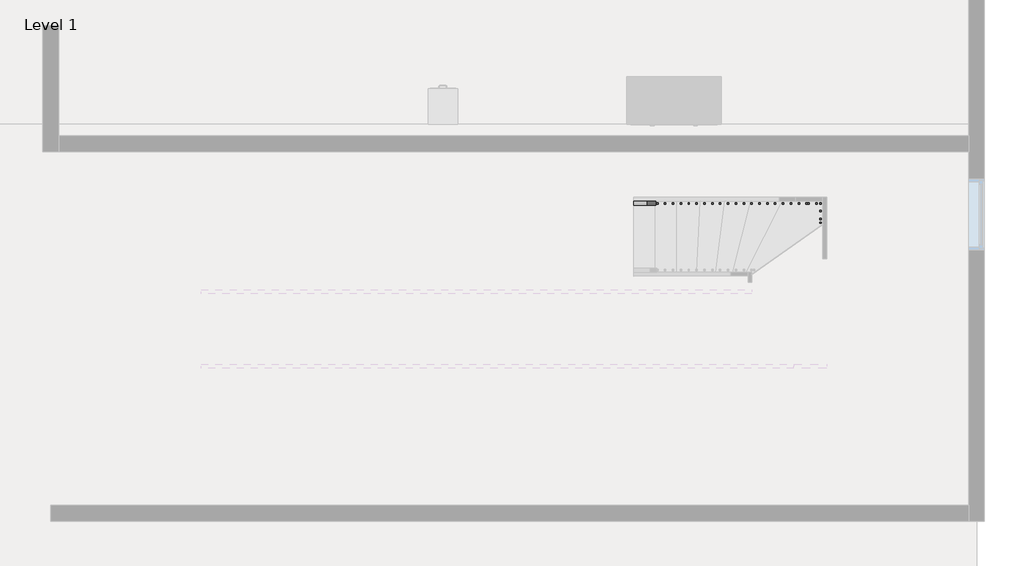
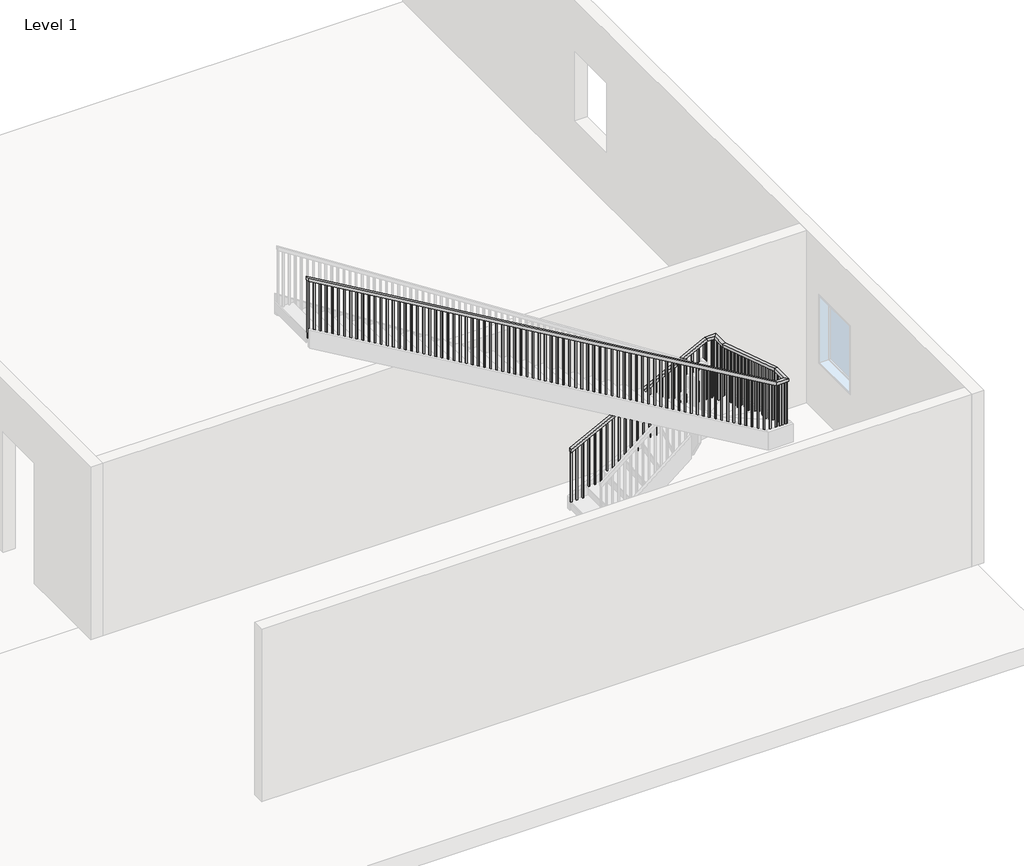
# One storey, part 3 of 4: 1 railing.
"""IFC4 building model written with IfcOpenShell, lengths in millimetres."""

from ifc_helpers import new_model, si_unit, frame, origin, place, context, project, spatial, polyline, outline, extrude, faceted_brep, element, save

model = new_model("IFC4")

# Units and contexts
model_context = context("Model", 3, world=origin())
ifc_project = project(units=[si_unit("LENGTHUNIT", "METRE", prefix="MILLI")], contexts=[model_context])

# Site, building, storey
site = spatial("IfcSite", under=ifc_project)
building = spatial("IfcBuilding", under=site)
storey = spatial("IfcBuildingStorey", under=building, Name="Level 1", Elevation=0.0)

# Railing
placement = place(None, origin())
element("IfcRailing", 1, ObjectType="Handrail - Rectangular", at=placement, inside=storey, context=model_context, shape_type="SolidModel", body=[
    faceted_brep([(11576.2992414, 971.4275916, 1109.0771751), (11576.2992414, 971.4275916, 1051.9280057), (11576.2992414, 920.6275916, 1051.9280057), (11576.2992414, 920.6275916, 1109.0771751), (13836.2810979, 971.4275916, 2273.7644996), (13848.6011492, 971.4275916, 2222.9644996), (13848.6011492, 920.6275916, 2222.9644996), (13836.2810979, 920.6275916, 2273.7644996), (14018.4309332, 971.4275916, 2273.7644996), (14018.4309332, 971.4275916, 2222.9644996), (13967.6309332, 920.6275916, 2222.9644996), (13967.6309332, 920.6275916, 2273.7644996), (14018.4309332, 694.273639, 2273.7644996), (14018.4309332, 686.3230629, 2222.9644996), (13967.6309332, 686.3230629, 2222.9644996), (13967.6309332, 694.273639, 2273.7644996), (14018.4309332, -805.6099604, 2755.0388853), (14018.4309332, -813.5605365, 2704.2388853), (13967.6309332, -813.5605365, 2704.2388853), (13967.6309332, -805.6099604, 2755.0388853), (14018.4309332, -1136.7724084, 2704.2388853), (14018.4309332, -1136.7724084, 2755.0388853), (13825.4484846, -1136.7724084, 2755.0388853), (13811.671706, -1136.7724084, 2704.2388853), (13967.6309332, -1085.9724084, 2704.2388853), (13811.671706, -1085.9724084, 2704.2388853), (13967.6309332, -1085.9724084, 2755.0388853), (13825.4484846, -1085.9724084, 2755.0388853), (5988.2992414, -1136.7724084, 7343.3084387), (5988.2992414, -1085.9724084, 7343.3084387), (5988.2992414, -1085.9724084, 7284.4428051), (5988.2992414, -1136.7724084, 7284.4428051)], [[[0, 1, 2, 3]], [[1, 0, 4, 5]], [[2, 1, 5, 6]], [[3, 2, 6, 7]], [[0, 3, 7, 4]], [[5, 4, 8, 9]], [[6, 5, 9, 10]], [[7, 6, 10, 11]], [[4, 7, 11, 8]], [[9, 8, 12, 13]], [[10, 9, 13, 14]], [[11, 10, 14, 15]], [[8, 11, 15, 12]], [[13, 12, 16, 17]], [[14, 13, 17, 18]], [[15, 14, 18, 19]], [[12, 15, 19, 16]], [[20, 21, 22, 23]], [[24, 20, 23, 25]], [[26, 24, 25, 27]], [[21, 26, 27, 22]], [[17, 16, 21, 20]], [[18, 17, 20, 24]], [[19, 18, 24, 26]], [[16, 19, 26, 21]], [[28, 29, 30, 31]], [[23, 22, 28, 31]], [[25, 23, 31, 30]], [[27, 25, 30, 29]], [[22, 27, 29, 28]]]),
    extrude(outline(polyline([(7281.852626, 5992.7234846), (6265.3333333, 5992.7234846), (6265.3333333, 6011.7734846), (7270.6997779, 6011.7734846), (7281.852626, 5992.7234846)])), frame((0.0, -1120.8974084, 0.0), z_axis=(0.0, 1.0, 0.0), x_axis=(0.0, 0.0, 1.0)), (0.0, 0.0, 1.0), 19.05),
    extrude(outline(polyline([(7222.3707695, 6094.3234846), (6265.3333333, 6094.3234846), (6265.3333333, 6113.3734846), (7211.2179214, 6113.3734846), (7222.3707695, 6094.3234846)])), frame((0.0, -1120.8974084, 0.0), z_axis=(0.0, 1.0, 0.0), x_axis=(0.0, 0.0, 1.0)), (0.0, 0.0, 1.0), 19.05),
    extrude(outline(polyline([(7162.888913, 6195.9234846), (6265.3333333, 6195.9234846), (6265.3333333, 6214.9734846), (7151.7360649, 6214.9734846), (7162.888913, 6195.9234846)])), frame((0.0, -1120.8974084, 0.0), z_axis=(0.0, 1.0, 0.0), x_axis=(0.0, 0.0, 1.0)), (0.0, 0.0, 1.0), 19.05),
    extrude(outline(polyline([(7103.4070565, 6297.5234846), (6096.0, 6297.5234846), (6096.0, 6316.5734846), (7092.2542084, 6316.5734846), (7103.4070565, 6297.5234846)])), frame((0.0, -1120.8974084, 0.0), z_axis=(0.0, 1.0, 0.0), x_axis=(0.0, 0.0, 1.0)), (0.0, 0.0, 1.0), 19.05),
    extrude(outline(polyline([(7043.9252, 6399.1234846), (6096.0, 6399.1234846), (6096.0, 6418.1734846), (7032.7723519, 6418.1734846), (7043.9252, 6399.1234846)])), frame((0.0, -1120.8974084, 0.0), z_axis=(0.0, 1.0, 0.0), x_axis=(0.0, 0.0, 1.0)), (0.0, 0.0, 1.0), 19.05),
    extrude(outline(polyline([(6984.4433435, 6500.7234846), (6096.0, 6500.7234846), (6096.0, 6519.7734846), (6973.2904954, 6519.7734846), (6984.4433435, 6500.7234846)])), frame((0.0, -1120.8974084, 0.0), z_axis=(0.0, 1.0, 0.0), x_axis=(0.0, 0.0, 1.0)), (0.0, 0.0, 1.0), 19.05),
    extrude(outline(polyline([(6924.961487, 6602.3234846), (5926.6666667, 6602.3234846), (5926.6666667, 6621.3734846), (6913.8086389, 6621.3734846), (6924.961487, 6602.3234846)])), frame((0.0, -1120.8974084, 0.0), z_axis=(0.0, 1.0, 0.0), x_axis=(0.0, 0.0, 1.0)), (0.0, 0.0, 1.0), 19.05),
    extrude(outline(polyline([(6865.4796305, 6703.9234846), (5926.6666667, 6703.9234846), (5926.6666667, 6722.9734846), (6854.3267824, 6722.9734846), (6865.4796305, 6703.9234846)])), frame((0.0, -1120.8974084, 0.0), z_axis=(0.0, 1.0, 0.0), x_axis=(0.0, 0.0, 1.0)), (0.0, 0.0, 1.0), 19.05),
    extrude(outline(polyline([(6805.997774, 6805.5234846), (5926.6666667, 6805.5234846), (5926.6666667, 6824.5734846), (6794.8449259, 6824.5734846), (6805.997774, 6805.5234846)])), frame((0.0, -1120.8974084, 0.0), z_axis=(0.0, 1.0, 0.0), x_axis=(0.0, 0.0, 1.0)), (0.0, 0.0, 1.0), 19.05),
    extrude(outline(polyline([(6746.5159175, 6907.1234846), (5757.3333333, 6907.1234846), (5757.3333333, 6926.1734846), (6735.3630694, 6926.1734846), (6746.5159175, 6907.1234846)])), frame((0.0, -1120.8974084, 0.0), z_axis=(0.0, 1.0, 0.0), x_axis=(0.0, 0.0, 1.0)), (0.0, 0.0, 1.0), 19.05),
    extrude(outline(polyline([(6687.034061, 7008.7234846), (5757.3333333, 7008.7234846), (5757.3333333, 7027.7734846), (6675.881213, 7027.7734846), (6687.034061, 7008.7234846)])), frame((0.0, -1120.8974084, 0.0), z_axis=(0.0, 1.0, 0.0), x_axis=(0.0, 0.0, 1.0)), (0.0, 0.0, 1.0), 19.05),
    extrude(outline(polyline([(6627.5522045, 7110.3234846), (5588.0, 7110.3234846), (5588.0, 7129.3734846), (6616.3993565, 7129.3734846), (6627.5522045, 7110.3234846)])), frame((0.0, -1120.8974084, 0.0), z_axis=(0.0, 1.0, 0.0), x_axis=(0.0, 0.0, 1.0)), (0.0, 0.0, 1.0), 19.05),
    extrude(outline(polyline([(6568.0703481, 7211.9234846), (5588.0, 7211.9234846), (5588.0, 7230.9734846), (6556.9175, 7230.9734846), (6568.0703481, 7211.9234846)])), frame((0.0, -1120.8974084, 0.0), z_axis=(0.0, 1.0, 0.0), x_axis=(0.0, 0.0, 1.0)), (0.0, 0.0, 1.0), 19.05),
    extrude(outline(polyline([(6508.5884916, 7313.5234846), (5588.0, 7313.5234846), (5588.0, 7332.5734846), (6497.4356435, 7332.5734846), (6508.5884916, 7313.5234846)])), frame((0.0, -1120.8974084, 0.0), z_axis=(0.0, 1.0, 0.0), x_axis=(0.0, 0.0, 1.0)), (0.0, 0.0, 1.0), 19.05),
    extrude(outline(polyline([(6449.1066351, 7415.1234846), (5418.6666667, 7415.1234846), (5418.6666667, 7434.1734846), (6437.953787, 7434.1734846), (6449.1066351, 7415.1234846)])), frame((0.0, -1120.8974084, 0.0), z_axis=(0.0, 1.0, 0.0), x_axis=(0.0, 0.0, 1.0)), (0.0, 0.0, 1.0), 19.05),
    extrude(outline(polyline([(6389.6247786, 7516.7234846), (5418.6666667, 7516.7234846), (5418.6666667, 7535.7734846), (6378.4719305, 7535.7734846), (6389.6247786, 7516.7234846)])), frame((0.0, -1120.8974084, 0.0), z_axis=(0.0, 1.0, 0.0), x_axis=(0.0, 0.0, 1.0)), (0.0, 0.0, 1.0), 19.05),
    extrude(outline(polyline([(6330.1429221, 7618.3234846), (5418.6666667, 7618.3234846), (5418.6666667, 7637.3734846), (6318.990074, 7637.3734846), (6330.1429221, 7618.3234846)])), frame((0.0, -1120.8974084, 0.0), z_axis=(0.0, 1.0, 0.0), x_axis=(0.0, 0.0, 1.0)), (0.0, 0.0, 1.0), 19.05),
    extrude(outline(polyline([(6270.6610656, 7719.9234846), (5249.3333333, 7719.9234846), (5249.3333333, 7738.9734846), (6259.5082175, 7738.9734846), (6270.6610656, 7719.9234846)])), frame((0.0, -1120.8974084, 0.0), z_axis=(0.0, 1.0, 0.0), x_axis=(0.0, 0.0, 1.0)), (0.0, 0.0, 1.0), 19.05),
    extrude(outline(polyline([(6211.1792091, 7821.5234846), (5249.3333333, 7821.5234846), (5249.3333333, 7840.5734846), (6200.026361, 7840.5734846), (6211.1792091, 7821.5234846)])), frame((0.0, -1120.8974084, 0.0), z_axis=(0.0, 1.0, 0.0), x_axis=(0.0, 0.0, 1.0)), (0.0, 0.0, 1.0), 19.05),
    extrude(outline(polyline([(6151.6973526, 7923.1234846), (5249.3333333, 7923.1234846), (5249.3333333, 7942.1734846), (6140.5445045, 7942.1734846), (6151.6973526, 7923.1234846)])), frame((0.0, -1120.8974084, 0.0), z_axis=(0.0, 1.0, 0.0), x_axis=(0.0, 0.0, 1.0)), (0.0, 0.0, 1.0), 19.05),
    extrude(outline(polyline([(6092.2154961, 8024.7234846), (5080.0, 8024.7234846), (5080.0, 8043.7734846), (6081.062648, 8043.7734846), (6092.2154961, 8024.7234846)])), frame((0.0, -1120.8974084, 0.0), z_axis=(0.0, 1.0, 0.0), x_axis=(0.0, 0.0, 1.0)), (0.0, 0.0, 1.0), 19.05),
    extrude(outline(polyline([(6032.7336396, 8126.3234846), (5080.0, 8126.3234846), (5080.0, 8145.3734846), (6021.5807915, 8145.3734846), (6032.7336396, 8126.3234846)])), frame((0.0, -1120.8974084, 0.0), z_axis=(0.0, 1.0, 0.0), x_axis=(0.0, 0.0, 1.0)), (0.0, 0.0, 1.0), 19.05),
    extrude(outline(polyline([(5973.2517831, 8227.9234846), (4910.6666667, 8227.9234846), (4910.6666667, 8246.9734846), (5962.098935, 8246.9734846), (5973.2517831, 8227.9234846)])), frame((0.0, -1120.8974084, 0.0), z_axis=(0.0, 1.0, 0.0), x_axis=(0.0, 0.0, 1.0)), (0.0, 0.0, 1.0), 19.05),
    extrude(outline(polyline([(5913.7699266, 8329.5234846), (4910.6666667, 8329.5234846), (4910.6666667, 8348.5734846), (5902.6170785, 8348.5734846), (5913.7699266, 8329.5234846)])), frame((0.0, -1120.8974084, 0.0), z_axis=(0.0, 1.0, 0.0), x_axis=(0.0, 0.0, 1.0)), (0.0, 0.0, 1.0), 19.05),
    extrude(outline(polyline([(5854.2880701, 8431.1234846), (4910.6666667, 8431.1234846), (4910.6666667, 8450.1734846), (5843.135222, 8450.1734846), (5854.2880701, 8431.1234846)])), frame((0.0, -1120.8974084, 0.0), z_axis=(0.0, 1.0, 0.0), x_axis=(0.0, 0.0, 1.0)), (0.0, 0.0, 1.0), 19.05),
    extrude(outline(polyline([(5794.8062136, 8532.7234846), (4741.3333333, 8532.7234846), (4741.3333333, 8551.7734846), (5783.6533655, 8551.7734846), (5794.8062136, 8532.7234846)])), frame((0.0, -1120.8974084, 0.0), z_axis=(0.0, 1.0, 0.0), x_axis=(0.0, 0.0, 1.0)), (0.0, 0.0, 1.0), 19.05),
    extrude(outline(polyline([(5735.3243571, 8634.3234846), (4741.3333333, 8634.3234846), (4741.3333333, 8653.3734846), (5724.171509, 8653.3734846), (5735.3243571, 8634.3234846)])), frame((0.0, -1120.8974084, 0.0), z_axis=(0.0, 1.0, 0.0), x_axis=(0.0, 0.0, 1.0)), (0.0, 0.0, 1.0), 19.05),
    extrude(outline(polyline([(5675.8425006, 8735.9234846), (4741.3333333, 8735.9234846), (4741.3333333, 8754.9734846), (5664.6896525, 8754.9734846), (5675.8425006, 8735.9234846)])), frame((0.0, -1120.8974084, 0.0), z_axis=(0.0, 1.0, 0.0), x_axis=(0.0, 0.0, 1.0)), (0.0, 0.0, 1.0), 19.05),
    extrude(outline(polyline([(5616.3606441, 8837.5234846), (4572.0, 8837.5234846), (4572.0, 8856.5734846), (5605.207796, 8856.5734846), (5616.3606441, 8837.5234846)])), frame((0.0, -1120.8974084, 0.0), z_axis=(0.0, 1.0, 0.0), x_axis=(0.0, 0.0, 1.0)), (0.0, 0.0, 1.0), 19.05),
    extrude(outline(polyline([(5556.8787876, 8939.1234846), (4572.0, 8939.1234846), (4572.0, 8958.1734846), (5545.7259395, 8958.1734846), (5556.8787876, 8939.1234846)])), frame((0.0, -1120.8974084, 0.0), z_axis=(0.0, 1.0, 0.0), x_axis=(0.0, 0.0, 1.0)), (0.0, 0.0, 1.0), 19.05),
    extrude(outline(polyline([(5497.3969311, 9040.7234846), (4572.0, 9040.7234846), (4572.0, 9059.7734846), (5486.244083, 9059.7734846), (5497.3969311, 9040.7234846)])), frame((0.0, -1120.8974084, 0.0), z_axis=(0.0, 1.0, 0.0), x_axis=(0.0, 0.0, 1.0)), (0.0, 0.0, 1.0), 19.05),
    extrude(outline(polyline([(5437.9150746, 9142.3234846), (4402.6666667, 9142.3234846), (4402.6666667, 9161.3734846), (5426.7622265, 9161.3734846), (5437.9150746, 9142.3234846)])), frame((0.0, -1120.8974084, 0.0), z_axis=(0.0, 1.0, 0.0), x_axis=(0.0, 0.0, 1.0)), (0.0, 0.0, 1.0), 19.05),
    extrude(outline(polyline([(5378.4332181, 9243.9234846), (4402.6666667, 9243.9234846), (4402.6666667, 9262.9734846), (5367.28037, 9262.9734846), (5378.4332181, 9243.9234846)])), frame((0.0, -1120.8974084, 0.0), z_axis=(0.0, 1.0, 0.0), x_axis=(0.0, 0.0, 1.0)), (0.0, 0.0, 1.0), 19.05),
    extrude(outline(polyline([(5318.9513616, 9345.5234846), (4233.3333333, 9345.5234846), (4233.3333333, 9364.5734846), (5307.7985135, 9364.5734846), (5318.9513616, 9345.5234846)])), frame((0.0, -1120.8974084, 0.0), z_axis=(0.0, 1.0, 0.0), x_axis=(0.0, 0.0, 1.0)), (0.0, 0.0, 1.0), 19.05),
    extrude(outline(polyline([(5259.4695051, 9447.1234846), (4233.3333333, 9447.1234846), (4233.3333333, 9466.1734846), (5248.316657, 9466.1734846), (5259.4695051, 9447.1234846)])), frame((0.0, -1120.8974084, 0.0), z_axis=(0.0, 1.0, 0.0), x_axis=(0.0, 0.0, 1.0)), (0.0, 0.0, 1.0), 19.05),
    extrude(outline(polyline([(5199.9876486, 9548.7234846), (4233.3333333, 9548.7234846), (4233.3333333, 9567.7734846), (5188.8348005, 9567.7734846), (5199.9876486, 9548.7234846)])), frame((0.0, -1120.8974084, 0.0), z_axis=(0.0, 1.0, 0.0), x_axis=(0.0, 0.0, 1.0)), (0.0, 0.0, 1.0), 19.05),
    extrude(outline(polyline([(5140.5057921, 9650.3234846), (4064.0, 9650.3234846), (4064.0, 9669.3734846), (5129.352944, 9669.3734846), (5140.5057921, 9650.3234846)])), frame((0.0, -1120.8974084, 0.0), z_axis=(0.0, 1.0, 0.0), x_axis=(0.0, 0.0, 1.0)), (0.0, 0.0, 1.0), 19.05),
    extrude(outline(polyline([(5081.0239356, 9751.9234846), (4064.0, 9751.9234846), (4064.0, 9770.9734846), (5069.8710875, 9770.9734846), (5081.0239356, 9751.9234846)])), frame((0.0, -1120.8974084, 0.0), z_axis=(0.0, 1.0, 0.0), x_axis=(0.0, 0.0, 1.0)), (0.0, 0.0, 1.0), 19.05),
    extrude(outline(polyline([(5021.5420791, 9853.5234846), (4064.0, 9853.5234846), (4064.0, 9872.5734846), (5010.389231, 9872.5734846), (5021.5420791, 9853.5234846)])), frame((0.0, -1120.8974084, 0.0), z_axis=(0.0, 1.0, 0.0), x_axis=(0.0, 0.0, 1.0)), (0.0, 0.0, 1.0), 19.05),
    extrude(outline(polyline([(4962.0602226, 9955.1234846), (3894.6666667, 9955.1234846), (3894.6666667, 9974.1734846), (4950.9073745, 9974.1734846), (4962.0602226, 9955.1234846)])), frame((0.0, -1120.8974084, 0.0), z_axis=(0.0, 1.0, 0.0), x_axis=(0.0, 0.0, 1.0)), (0.0, 0.0, 1.0), 19.05),
    extrude(outline(polyline([(4902.5783661, 10056.7234846), (3894.6666667, 10056.7234846), (3894.6666667, 10075.7734846), (4891.4255181, 10075.7734846), (4902.5783661, 10056.7234846)])), frame((0.0, -1120.8974084, 0.0), z_axis=(0.0, 1.0, 0.0), x_axis=(0.0, 0.0, 1.0)), (0.0, 0.0, 1.0), 19.05),
    extrude(outline(polyline([(4843.0965096, 10158.3234846), (3894.6666667, 10158.3234846), (3894.6666667, 10177.3734846), (4831.9436616, 10177.3734846), (4843.0965096, 10158.3234846)])), frame((0.0, -1120.8974084, 0.0), z_axis=(0.0, 1.0, 0.0), x_axis=(0.0, 0.0, 1.0)), (0.0, 0.0, 1.0), 19.05),
    extrude(outline(polyline([(4783.6146532, 10259.9234846), (3725.3333333, 10259.9234846), (3725.3333333, 10278.9734846), (4772.4618051, 10278.9734846), (4783.6146532, 10259.9234846)])), frame((0.0, -1120.8974084, 0.0), z_axis=(0.0, 1.0, 0.0), x_axis=(0.0, 0.0, 1.0)), (0.0, 0.0, 1.0), 19.05),
    extrude(outline(polyline([(4724.1327967, 10361.5234846), (3725.3333333, 10361.5234846), (3725.3333333, 10380.5734846), (4712.9799486, 10380.5734846), (4724.1327967, 10361.5234846)])), frame((0.0, -1120.8974084, 0.0), z_axis=(0.0, 1.0, 0.0), x_axis=(0.0, 0.0, 1.0)), (0.0, 0.0, 1.0), 19.05),
    extrude(outline(polyline([(4664.6509402, 10463.1234846), (3725.3333333, 10463.1234846), (3725.3333333, 10482.1734846), (4653.4980921, 10482.1734846), (4664.6509402, 10463.1234846)])), frame((0.0, -1120.8974084, 0.0), z_axis=(0.0, 1.0, 0.0), x_axis=(0.0, 0.0, 1.0)), (0.0, 0.0, 1.0), 19.05),
    extrude(outline(polyline([(4605.1690837, 10564.7234846), (3556.0, 10564.7234846), (3556.0, 10583.7734846), (4594.0162356, 10583.7734846), (4605.1690837, 10564.7234846)])), frame((0.0, -1120.8974084, 0.0), z_axis=(0.0, 1.0, 0.0), x_axis=(0.0, 0.0, 1.0)), (0.0, 0.0, 1.0), 19.05),
    extrude(outline(polyline([(4545.6872272, 10666.3234846), (3556.0, 10666.3234846), (3556.0, 10685.3734846), (4534.5343791, 10685.3734846), (4545.6872272, 10666.3234846)])), frame((0.0, -1120.8974084, 0.0), z_axis=(0.0, 1.0, 0.0), x_axis=(0.0, 0.0, 1.0)), (0.0, 0.0, 1.0), 19.05),
    extrude(outline(polyline([(4486.2053707, 10767.9234846), (3386.6666667, 10767.9234846), (3386.6666667, 10786.9734846), (4475.0525226, 10786.9734846), (4486.2053707, 10767.9234846)])), frame((0.0, -1120.8974084, 0.0), z_axis=(0.0, 1.0, 0.0), x_axis=(0.0, 0.0, 1.0)), (0.0, 0.0, 1.0), 19.05),
    extrude(outline(polyline([(4426.7235142, 10869.5234846), (3386.6666667, 10869.5234846), (3386.6666667, 10888.5734846), (4415.5706661, 10888.5734846), (4426.7235142, 10869.5234846)])), frame((0.0, -1120.8974084, 0.0), z_axis=(0.0, 1.0, 0.0), x_axis=(0.0, 0.0, 1.0)), (0.0, 0.0, 1.0), 19.05),
    extrude(outline(polyline([(4367.2416577, 10971.1234846), (3386.6666667, 10971.1234846), (3386.6666667, 10990.1734846), (4356.0888096, 10990.1734846), (4367.2416577, 10971.1234846)])), frame((0.0, -1120.8974084, 0.0), z_axis=(0.0, 1.0, 0.0), x_axis=(0.0, 0.0, 1.0)), (0.0, 0.0, 1.0), 19.05),
    extrude(outline(polyline([(4307.7598012, 11072.7234846), (3217.3333333, 11072.7234846), (3217.3333333, 11091.7734846), (4296.6069531, 11091.7734846), (4307.7598012, 11072.7234846)])), frame((0.0, -1120.8974084, 0.0), z_axis=(0.0, 1.0, 0.0), x_axis=(0.0, 0.0, 1.0)), (0.0, 0.0, 1.0), 19.05),
    extrude(outline(polyline([(4248.2779447, 11174.3234846), (3217.3333333, 11174.3234846), (3217.3333333, 11193.3734846), (4237.1250966, 11193.3734846), (4248.2779447, 11174.3234846)])), frame((0.0, -1120.8974084, 0.0), z_axis=(0.0, 1.0, 0.0), x_axis=(0.0, 0.0, 1.0)), (0.0, 0.0, 1.0), 19.05),
    extrude(outline(polyline([(4188.7960882, 11275.9234846), (3217.3333333, 11275.9234846), (3217.3333333, 11294.9734846), (4177.6432401, 11294.9734846), (4188.7960882, 11275.9234846)])), frame((0.0, -1120.8974084, 0.0), z_axis=(0.0, 1.0, 0.0), x_axis=(0.0, 0.0, 1.0)), (0.0, 0.0, 1.0), 19.05),
    extrude(outline(polyline([(4129.3142317, 11377.5234846), (3048.0, 11377.5234846), (3048.0, 11396.5734846), (4118.1613836, 11396.5734846), (4129.3142317, 11377.5234846)])), frame((0.0, -1120.8974084, 0.0), z_axis=(0.0, 1.0, 0.0), x_axis=(0.0, 0.0, 1.0)), (0.0, 0.0, 1.0), 19.05),
    extrude(outline(polyline([(4069.8323752, 11479.1234846), (3048.0, 11479.1234846), (3048.0, 11498.1734846), (4058.6795271, 11498.1734846), (4069.8323752, 11479.1234846)])), frame((0.0, -1120.8974084, 0.0), z_axis=(0.0, 1.0, 0.0), x_axis=(0.0, 0.0, 1.0)), (0.0, 0.0, 1.0), 19.05),
    extrude(outline(polyline([(4010.3505187, 11580.7234846), (3048.0, 11580.7234846), (3048.0, 11599.7734846), (3999.1976706, 11599.7734846), (4010.3505187, 11580.7234846)])), frame((0.0, -1120.8974084, 0.0), z_axis=(0.0, 1.0, 0.0), x_axis=(0.0, 0.0, 1.0)), (0.0, 0.0, 1.0), 19.05),
    extrude(outline(polyline([(3950.8686622, 11682.3234846), (2878.6666667, 11682.3234846), (2878.6666667, 11701.3734846), (3939.7158141, 11701.3734846), (3950.8686622, 11682.3234846)])), frame((0.0, -1120.8974084, 0.0), z_axis=(0.0, 1.0, 0.0), x_axis=(0.0, 0.0, 1.0)), (0.0, 0.0, 1.0), 19.05),
    extrude(outline(polyline([(3891.3868057, 11783.9234846), (2878.6666667, 11783.9234846), (2878.6666667, 11802.9734846), (3880.2339576, 11802.9734846), (3891.3868057, 11783.9234846)])), frame((0.0, -1120.8974084, 0.0), z_axis=(0.0, 1.0, 0.0), x_axis=(0.0, 0.0, 1.0)), (0.0, 0.0, 1.0), 19.05),
    extrude(outline(polyline([(3831.9049492, 11885.5234846), (2878.6666667, 11885.5234846), (2878.6666667, 11904.5734846), (3820.7521011, 11904.5734846), (3831.9049492, 11885.5234846)])), frame((0.0, -1120.8974084, 0.0), z_axis=(0.0, 1.0, 0.0), x_axis=(0.0, 0.0, 1.0)), (0.0, 0.0, 1.0), 19.05),
    extrude(outline(polyline([(3772.4230927, 11987.1234846), (2709.3333333, 11987.1234846), (2709.3333333, 12006.1734846), (3761.2702446, 12006.1734846), (3772.4230927, 11987.1234846)])), frame((0.0, -1120.8974084, 0.0), z_axis=(0.0, 1.0, 0.0), x_axis=(0.0, 0.0, 1.0)), (0.0, 0.0, 1.0), 19.05),
    extrude(outline(polyline([(3712.9412362, 12088.7234846), (2709.3333333, 12088.7234846), (2709.3333333, 12107.7734846), (3701.7883881, 12107.7734846), (3712.9412362, 12088.7234846)])), frame((0.0, -1120.8974084, 0.0), z_axis=(0.0, 1.0, 0.0), x_axis=(0.0, 0.0, 1.0)), (0.0, 0.0, 1.0), 19.05),
    extrude(outline(polyline([(3653.4593797, 12190.3234846), (2540.0, 12190.3234846), (2540.0, 12209.3734846), (3642.3065316, 12209.3734846), (3653.4593797, 12190.3234846)])), frame((0.0, -1120.8974084, 0.0), z_axis=(0.0, 1.0, 0.0), x_axis=(0.0, 0.0, 1.0)), (0.0, 0.0, 1.0), 19.05),
    extrude(outline(polyline([(3593.9775232, 12291.9234846), (2540.0, 12291.9234846), (2540.0, 12310.9734846), (3582.8246751, 12310.9734846), (3593.9775232, 12291.9234846)])), frame((0.0, -1120.8974084, 0.0), z_axis=(0.0, 1.0, 0.0), x_axis=(0.0, 0.0, 1.0)), (0.0, 0.0, 1.0), 19.05),
    extrude(outline(polyline([(3534.4956667, 12393.5234846), (2540.0, 12393.5234846), (2540.0, 12412.5734846), (3523.3428186, 12412.5734846), (3534.4956667, 12393.5234846)])), frame((0.0, -1120.8974084, 0.0), z_axis=(0.0, 1.0, 0.0), x_axis=(0.0, 0.0, 1.0)), (0.0, 0.0, 1.0), 19.05),
    extrude(outline(polyline([(3475.0138102, 12495.1234846), (2370.6666667, 12495.1234846), (2370.6666667, 12514.1734846), (3463.8609621, 12514.1734846), (3475.0138102, 12495.1234846)])), frame((0.0, -1120.8974084, 0.0), z_axis=(0.0, 1.0, 0.0), x_axis=(0.0, 0.0, 1.0)), (0.0, 0.0, 1.0), 19.05),
    extrude(outline(polyline([(3415.5319537, 12596.7234846), (2370.6666667, 12596.7234846), (2370.6666667, 12615.7734846), (3404.3791056, 12615.7734846), (3415.5319537, 12596.7234846)])), frame((0.0, -1120.8974084, 0.0), z_axis=(0.0, 1.0, 0.0), x_axis=(0.0, 0.0, 1.0)), (0.0, 0.0, 1.0), 19.05),
    extrude(outline(polyline([(3356.0500972, 12698.3234846), (2370.6666667, 12698.3234846), (2370.6666667, 12717.3734846), (3344.8972491, 12717.3734846), (3356.0500972, 12698.3234846)])), frame((0.0, -1120.8974084, 0.0), z_axis=(0.0, 1.0, 0.0), x_axis=(0.0, 0.0, 1.0)), (0.0, 0.0, 1.0), 19.05),
    extrude(outline(polyline([(3296.5682407, 12799.9234846), (2201.3333333, 12799.9234846), (2201.3333333, 12818.9734846), (3285.4153926, 12818.9734846), (3296.5682407, 12799.9234846)])), frame((0.0, -1120.8974084, 0.0), z_axis=(0.0, 1.0, 0.0), x_axis=(0.0, 0.0, 1.0)), (0.0, 0.0, 1.0), 19.05),
    extrude(outline(polyline([(3237.0863842, 12901.5234846), (2201.3333333, 12901.5234846), (2201.3333333, 12920.5734846), (3225.9335361, 12920.5734846), (3237.0863842, 12901.5234846)])), frame((0.0, -1120.8974084, 0.0), z_axis=(0.0, 1.0, 0.0), x_axis=(0.0, 0.0, 1.0)), (0.0, 0.0, 1.0), 19.05),
    extrude(outline(polyline([(3177.6045277, 13003.1234846), (2201.3333333, 13003.1234846), (2201.3333333, 13022.1734846), (3166.4516796, 13022.1734846), (3177.6045277, 13003.1234846)])), frame((0.0, -1120.8974084, 0.0), z_axis=(0.0, 1.0, 0.0), x_axis=(0.0, 0.0, 1.0)), (0.0, 0.0, 1.0), 19.05),
    extrude(outline(polyline([(3118.1226712, 13104.7234846), (2032.0, 13104.7234846), (2032.0, 13123.7734846), (3106.9698231, 13123.7734846), (3118.1226712, 13104.7234846)])), frame((0.0, -1120.8974084, 0.0), z_axis=(0.0, 1.0, 0.0), x_axis=(0.0, 0.0, 1.0)), (0.0, 0.0, 1.0), 19.05),
    extrude(outline(polyline([(3058.6408147, 13206.3234846), (2032.0, 13206.3234846), (2032.0, 13225.3734846), (3047.4879667, 13225.3734846), (3058.6408147, 13206.3234846)])), frame((0.0, -1120.8974084, 0.0), z_axis=(0.0, 1.0, 0.0), x_axis=(0.0, 0.0, 1.0)), (0.0, 0.0, 1.0), 19.05),
    extrude(outline(polyline([(2999.1589582, 13307.9234846), (2032.0, 13307.9234846), (2032.0, 13326.9734846), (2988.0061102, 13326.9734846), (2999.1589582, 13307.9234846)])), frame((0.0, -1120.8974084, 0.0), z_axis=(0.0, 1.0, 0.0), x_axis=(0.0, 0.0, 1.0)), (0.0, 0.0, 1.0), 19.05),
    extrude(outline(polyline([(2939.6771018, 13409.5234846), (2032.0, 13409.5234846), (2032.0, 13428.5734846), (2928.5242537, 13428.5734846), (2939.6771018, 13409.5234846)])), frame((0.0, -1120.8974084, 0.0), z_axis=(0.0, 1.0, 0.0), x_axis=(0.0, 0.0, 1.0)), (0.0, 0.0, 1.0), 19.05),
    extrude(outline(polyline([(2880.1952453, 13511.1234846), (1862.6666667, 13511.1234846), (1862.6666667, 13530.1734846), (2869.0423972, 13530.1734846), (2880.1952453, 13511.1234846)])), frame((0.0, -1120.8974084, 0.0), z_axis=(0.0, 1.0, 0.0), x_axis=(0.0, 0.0, 1.0)), (0.0, 0.0, 1.0), 19.05),
    extrude(outline(polyline([(2820.7133888, 13612.7234846), (1862.6666667, 13612.7234846), (1862.6666667, 13631.7734846), (2809.5605407, 13631.7734846), (2820.7133888, 13612.7234846)])), frame((0.0, -1120.8974084, 0.0), z_axis=(0.0, 1.0, 0.0), x_axis=(0.0, 0.0, 1.0)), (0.0, 0.0, 1.0), 19.05),
    extrude(outline(polyline([(2761.2315323, 13714.3234846), (1862.6666667, 13714.3234846), (1862.6666667, 13733.3734846), (2750.0786842, 13733.3734846), (2761.2315323, 13714.3234846)])), frame((0.0, -1120.8974084, 0.0), z_axis=(0.0, 1.0, 0.0), x_axis=(0.0, 0.0, 1.0)), (0.0, 0.0, 1.0), 19.05),
    extrude(outline(polyline([(13900.9559332, -1120.8974084), (13881.9059332, -1120.8974084), (13881.9059332, -1101.8474084), (13900.9559332, -1101.8474084), (13900.9559332, -1120.8974084)])), frame((0.0, 0.0, 1862.6666667), z_axis=(0.0, 0.0, 1.0), x_axis=(1.0, 0.0, 0.0)), (0.0, 0.0, 1.0), 841.5722186),
    extrude(outline(polyline([(14002.5559332, -1100.8849604), (14002.5559332, -1119.9349604), (13983.5059332, -1119.9349604), (13983.5059332, -1100.8849604), (14002.5559332, -1100.8849604)])), frame((0.0, 0.0, 1862.6666667), z_axis=(0.0, 0.0, 1.0), x_axis=(1.0, 0.0, 0.0)), (0.0, 0.0, 1.0), 841.5722186),
    extrude(outline(polyline([(14002.5559332, -999.2849604), (14002.5559332, -1018.3349604), (13983.5059332, -1018.3349604), (13983.5059332, -999.2849604), (14002.5559332, -999.2849604)])), frame((0.0, 0.0, 1862.6666667), z_axis=(0.0, 0.0, 1.0), x_axis=(1.0, 0.0, 0.0)), (0.0, 0.0, 1.0), 841.5722186),
    extrude(outline(polyline([(14002.5559332, -897.6849604), (14002.5559332, -916.7349604), (13983.5059332, -916.7349604), (13983.5059332, -897.6849604), (14002.5559332, -897.6849604)])), frame((0.0, 0.0, 1862.6666667), z_axis=(0.0, 0.0, 1.0), x_axis=(1.0, 0.0, 0.0)), (0.0, 0.0, 1.0), 841.5722186),
    extrude(outline(polyline([(-718.601361, 2673.7689082), (-718.601361, 1693.3333333), (-737.651361, 1693.3333333), (-737.651361, 2679.8815673), (-718.601361, 2673.7689082)])), frame((13983.5059332, 0.0, 0.0), z_axis=(1.0, 0.0, 0.0), x_axis=(0.0, 1.0, 0.0)), (0.0, 0.0, 1.0), 19.05),
    extrude(outline(polyline([(-617.001361, 2641.16806), (-617.001361, 1693.3333333), (-636.051361, 1693.3333333), (-636.051361, 2647.280719), (-617.001361, 2641.16806)])), frame((13983.5059332, 0.0, 0.0), z_axis=(1.0, 0.0, 0.0), x_axis=(0.0, 1.0, 0.0)), (0.0, 0.0, 1.0), 19.05),
    extrude(outline(polyline([(-515.401361, 2608.5672118), (-515.401361, 1693.3333333), (-534.451361, 1693.3333333), (-534.451361, 2614.6798708), (-515.401361, 2608.5672118)])), frame((13983.5059332, 0.0, 0.0), z_axis=(1.0, 0.0, 0.0), x_axis=(0.0, 1.0, 0.0)), (0.0, 0.0, 1.0), 19.05),
    extrude(outline(polyline([(-413.801361, 2575.9663635), (-413.801361, 1693.3333333), (-432.851361, 1693.3333333), (-432.851361, 2582.0790226), (-413.801361, 2575.9663635)])), frame((13983.5059332, 0.0, 0.0), z_axis=(1.0, 0.0, 0.0), x_axis=(0.0, 1.0, 0.0)), (0.0, 0.0, 1.0), 19.05),
    extrude(outline(polyline([(-312.201361, 2543.3655153), (-312.201361, 1693.3333333), (-331.251361, 1693.3333333), (-331.251361, 2549.4781744), (-312.201361, 2543.3655153)])), frame((13983.5059332, 0.0, 0.0), z_axis=(1.0, 0.0, 0.0), x_axis=(0.0, 1.0, 0.0)), (0.0, 0.0, 1.0), 19.05),
    extrude(outline(polyline([(-210.601361, 2510.7646671), (-210.601361, 1524.0), (-229.651361, 1524.0), (-229.651361, 2516.8773261), (-210.601361, 2510.7646671)])), frame((13983.5059332, 0.0, 0.0), z_axis=(1.0, 0.0, 0.0), x_axis=(0.0, 1.0, 0.0)), (0.0, 0.0, 1.0), 19.05),
    extrude(outline(polyline([(-109.001361, 2478.1638189), (-109.001361, 1524.0), (-128.051361, 1524.0), (-128.051361, 2484.2764779), (-109.001361, 2478.1638189)])), frame((13983.5059332, 0.0, 0.0), z_axis=(1.0, 0.0, 0.0), x_axis=(0.0, 1.0, 0.0)), (0.0, 0.0, 1.0), 19.05),
    extrude(outline(polyline([(-7.401361, 2445.5629706), (-7.401361, 1524.0), (-26.451361, 1524.0), (-26.451361, 2451.6756297), (-7.401361, 2445.5629706)])), frame((13983.5059332, 0.0, 0.0), z_axis=(1.0, 0.0, 0.0), x_axis=(0.0, 1.0, 0.0)), (0.0, 0.0, 1.0), 19.05),
    extrude(outline(polyline([(94.198639, 2412.9621224), (94.198639, 1524.0), (75.148639, 1524.0), (75.148639, 2419.0747814), (94.198639, 2412.9621224)])), frame((13983.5059332, 0.0, 0.0), z_axis=(1.0, 0.0, 0.0), x_axis=(0.0, 1.0, 0.0)), (0.0, 0.0, 1.0), 19.05),
    extrude(outline(polyline([(195.798639, 2380.3612742), (195.798639, 1354.6666667), (176.748639, 1354.6666667), (176.748639, 2386.4739332), (195.798639, 2380.3612742)])), frame((13983.5059332, 0.0, 0.0), z_axis=(1.0, 0.0, 0.0), x_axis=(0.0, 1.0, 0.0)), (0.0, 0.0, 1.0), 19.05),
    extrude(outline(polyline([(297.398639, 2347.7604259), (297.398639, 1354.6666667), (278.348639, 1354.6666667), (278.348639, 2353.873085), (297.398639, 2347.7604259)])), frame((13983.5059332, 0.0, 0.0), z_axis=(1.0, 0.0, 0.0), x_axis=(0.0, 1.0, 0.0)), (0.0, 0.0, 1.0), 19.05),
    extrude(outline(polyline([(398.998639, 2315.1595777), (398.998639, 1354.6666667), (379.948639, 1354.6666667), (379.948639, 2321.2722368), (398.998639, 2315.1595777)])), frame((13983.5059332, 0.0, 0.0), z_axis=(1.0, 0.0, 0.0), x_axis=(0.0, 1.0, 0.0)), (0.0, 0.0, 1.0), 19.05),
    extrude(outline(polyline([(500.598639, 2282.5587295), (500.598639, 1354.6666667), (481.548639, 1354.6666667), (481.548639, 2288.6713885), (500.598639, 2282.5587295)])), frame((13983.5059332, 0.0, 0.0), z_axis=(1.0, 0.0, 0.0), x_axis=(0.0, 1.0, 0.0)), (0.0, 0.0, 1.0), 19.05),
    extrude(outline(polyline([(602.198639, 2249.9578813), (602.198639, 1354.6666667), (583.148639, 1354.6666667), (583.148639, 2256.0705403), (602.198639, 2249.9578813)])), frame((13983.5059332, 0.0, 0.0), z_axis=(1.0, 0.0, 0.0), x_axis=(0.0, 1.0, 0.0)), (0.0, 0.0, 1.0), 19.05),
    extrude(outline(polyline([(14002.5559332, 752.3525916), (14002.5559332, 733.3025916), (13983.5059332, 733.3025916), (13983.5059332, 752.3525916), (14002.5559332, 752.3525916)])), frame((0.0, 0.0, 1185.3333333), z_axis=(0.0, 0.0, 1.0), x_axis=(1.0, 0.0, 0.0)), (0.0, 0.0, 1.0), 1037.6311663),
    extrude(outline(polyline([(14002.5559332, 853.9525916), (14002.5559332, 834.9025916), (13983.5059332, 834.9025916), (13983.5059332, 853.9525916), (14002.5559332, 853.9525916)])), frame((0.0, 0.0, 1185.3333333), z_axis=(0.0, 0.0, 1.0), x_axis=(1.0, 0.0, 0.0)), (0.0, 0.0, 1.0), 1037.6311663),
    extrude(outline(polyline([(13928.3560979, 955.5525916), (13947.4060979, 955.5525916), (13947.4060979, 936.5025916), (13928.3560979, 936.5025916), (13928.3560979, 955.5525916)])), frame((0.0, 0.0, 1185.3333333), z_axis=(0.0, 0.0, 1.0), x_axis=(1.0, 0.0, 0.0)), (0.0, 0.0, 1.0), 1037.6311663),
    extrude(outline(polyline([(2198.9352056, 13801.9742414), (1185.3333333, 13801.9742414), (1185.3333333, 13821.0242414), (2208.752671, 13821.0242414), (2198.9352056, 13801.9742414)])), frame((0.0, 936.5025916, 0.0), z_axis=(0.0, 1.0, 0.0), x_axis=(0.0, 0.0, 1.0)), (0.0, 0.0, 1.0), 19.05),
    extrude(outline(polyline([(2146.5753905, 13700.3742414), (1185.3333333, 13700.3742414), (1185.3333333, 13719.4242414), (2156.3928558, 13719.4242414), (2146.5753905, 13700.3742414)])), frame((0.0, 936.5025916, 0.0), z_axis=(0.0, 1.0, 0.0), x_axis=(0.0, 0.0, 1.0)), (0.0, 0.0, 1.0), 19.05),
    extrude(outline(polyline([(2094.2155754, 13598.7742414), (1185.3333333, 13598.7742414), (1185.3333333, 13617.8242414), (2104.0330407, 13617.8242414), (2094.2155754, 13598.7742414)])), frame((0.0, 936.5025916, 0.0), z_axis=(0.0, 1.0, 0.0), x_axis=(0.0, 0.0, 1.0)), (0.0, 0.0, 1.0), 19.05),
    extrude(outline(polyline([(2041.8557603, 13497.1742414), (1185.3333333, 13497.1742414), (1185.3333333, 13516.2242414), (2051.6732256, 13516.2242414), (2041.8557603, 13497.1742414)])), frame((0.0, 936.5025916, 0.0), z_axis=(0.0, 1.0, 0.0), x_axis=(0.0, 0.0, 1.0)), (0.0, 0.0, 1.0), 19.05),
    extrude(outline(polyline([(1989.4959452, 13395.5742414), (1016.0, 13395.5742414), (1016.0, 13414.6242414), (1999.3134105, 13414.6242414), (1989.4959452, 13395.5742414)])), frame((0.0, 936.5025916, 0.0), z_axis=(0.0, 1.0, 0.0), x_axis=(0.0, 0.0, 1.0)), (0.0, 0.0, 1.0), 19.05),
    extrude(outline(polyline([(1937.13613, 13293.9742414), (1016.0, 13293.9742414), (1016.0, 13313.0242414), (1946.9535954, 13313.0242414), (1937.13613, 13293.9742414)])), frame((0.0, 936.5025916, 0.0), z_axis=(0.0, 1.0, 0.0), x_axis=(0.0, 0.0, 1.0)), (0.0, 0.0, 1.0), 19.05),
    extrude(outline(polyline([(1884.7763149, 13192.3742414), (1016.0, 13192.3742414), (1016.0, 13211.4242414), (1894.5937803, 13211.4242414), (1884.7763149, 13192.3742414)])), frame((0.0, 936.5025916, 0.0), z_axis=(0.0, 1.0, 0.0), x_axis=(0.0, 0.0, 1.0)), (0.0, 0.0, 1.0), 19.05),
    extrude(outline(polyline([(1832.4164998, 13090.7742414), (1016.0, 13090.7742414), (1016.0, 13109.8242414), (1842.2339651, 13109.8242414), (1832.4164998, 13090.7742414)])), frame((0.0, 936.5025916, 0.0), z_axis=(0.0, 1.0, 0.0), x_axis=(0.0, 0.0, 1.0)), (0.0, 0.0, 1.0), 19.05),
    extrude(outline(polyline([(1780.0566847, 12989.1742414), (846.6666667, 12989.1742414), (846.6666667, 13008.2242414), (1789.87415, 13008.2242414), (1780.0566847, 12989.1742414)])), frame((0.0, 936.5025916, 0.0), z_axis=(0.0, 1.0, 0.0), x_axis=(0.0, 0.0, 1.0)), (0.0, 0.0, 1.0), 19.05),
    extrude(outline(polyline([(1727.6968696, 12887.5742414), (846.6666667, 12887.5742414), (846.6666667, 12906.6242414), (1737.5143349, 12906.6242414), (1727.6968696, 12887.5742414)])), frame((0.0, 936.5025916, 0.0), z_axis=(0.0, 1.0, 0.0), x_axis=(0.0, 0.0, 1.0)), (0.0, 0.0, 1.0), 19.05),
    extrude(outline(polyline([(1675.3370545, 12785.9742414), (846.6666667, 12785.9742414), (846.6666667, 12805.0242414), (1685.1545198, 12805.0242414), (1675.3370545, 12785.9742414)])), frame((0.0, 936.5025916, 0.0), z_axis=(0.0, 1.0, 0.0), x_axis=(0.0, 0.0, 1.0)), (0.0, 0.0, 1.0), 19.05),
    extrude(outline(polyline([(1622.9772393, 12684.3742414), (677.3333333, 12684.3742414), (677.3333333, 12703.4242414), (1632.7947047, 12703.4242414), (1622.9772393, 12684.3742414)])), frame((0.0, 936.5025916, 0.0), z_axis=(0.0, 1.0, 0.0), x_axis=(0.0, 0.0, 1.0)), (0.0, 0.0, 1.0), 19.05),
    extrude(outline(polyline([(1570.6174242, 12582.7742414), (677.3333333, 12582.7742414), (677.3333333, 12601.8242414), (1580.4348896, 12601.8242414), (1570.6174242, 12582.7742414)])), frame((0.0, 936.5025916, 0.0), z_axis=(0.0, 1.0, 0.0), x_axis=(0.0, 0.0, 1.0)), (0.0, 0.0, 1.0), 19.05),
    extrude(outline(polyline([(1518.2576091, 12481.1742414), (677.3333333, 12481.1742414), (677.3333333, 12500.2242414), (1528.0750744, 12500.2242414), (1518.2576091, 12481.1742414)])), frame((0.0, 936.5025916, 0.0), z_axis=(0.0, 1.0, 0.0), x_axis=(0.0, 0.0, 1.0)), (0.0, 0.0, 1.0), 19.05),
    extrude(outline(polyline([(1465.897794, 12379.5742414), (508.0, 12379.5742414), (508.0, 12398.6242414), (1475.7152593, 12398.6242414), (1465.897794, 12379.5742414)])), frame((0.0, 936.5025916, 0.0), z_axis=(0.0, 1.0, 0.0), x_axis=(0.0, 0.0, 1.0)), (0.0, 0.0, 1.0), 19.05),
    extrude(outline(polyline([(1413.5379789, 12277.9742414), (508.0, 12277.9742414), (508.0, 12297.0242414), (1423.3554442, 12297.0242414), (1413.5379789, 12277.9742414)])), frame((0.0, 936.5025916, 0.0), z_axis=(0.0, 1.0, 0.0), x_axis=(0.0, 0.0, 1.0)), (0.0, 0.0, 1.0), 19.05),
    extrude(outline(polyline([(1361.1781638, 12176.3742414), (508.0, 12176.3742414), (508.0, 12195.4242414), (1370.9956291, 12195.4242414), (1361.1781638, 12176.3742414)])), frame((0.0, 936.5025916, 0.0), z_axis=(0.0, 1.0, 0.0), x_axis=(0.0, 0.0, 1.0)), (0.0, 0.0, 1.0), 19.05),
    extrude(outline(polyline([(1308.8183486, 12074.7742414), (338.6666667, 12074.7742414), (338.6666667, 12093.8242414), (1318.635814, 12093.8242414), (1308.8183486, 12074.7742414)])), frame((0.0, 936.5025916, 0.0), z_axis=(0.0, 1.0, 0.0), x_axis=(0.0, 0.0, 1.0)), (0.0, 0.0, 1.0), 19.05),
    extrude(outline(polyline([(1256.4585335, 11973.1742414), (338.6666667, 11973.1742414), (338.6666667, 11992.2242414), (1266.2759989, 11992.2242414), (1256.4585335, 11973.1742414)])), frame((0.0, 936.5025916, 0.0), z_axis=(0.0, 1.0, 0.0), x_axis=(0.0, 0.0, 1.0)), (0.0, 0.0, 1.0), 19.05),
    extrude(outline(polyline([(1204.0987184, 11871.5742414), (338.6666667, 11871.5742414), (338.6666667, 11890.6242414), (1213.9161837, 11890.6242414), (1204.0987184, 11871.5742414)])), frame((0.0, 936.5025916, 0.0), z_axis=(0.0, 1.0, 0.0), x_axis=(0.0, 0.0, 1.0)), (0.0, 0.0, 1.0), 19.05),
    extrude(outline(polyline([(1151.7389033, 11769.9742414), (169.3333333, 11769.9742414), (169.3333333, 11789.0242414), (1161.5563686, 11789.0242414), (1151.7389033, 11769.9742414)])), frame((0.0, 936.5025916, 0.0), z_axis=(0.0, 1.0, 0.0), x_axis=(0.0, 0.0, 1.0)), (0.0, 0.0, 1.0), 19.05),
    extrude(outline(polyline([(1099.3790882, 11668.3742414), (169.3333333, 11668.3742414), (169.3333333, 11687.4242414), (1109.1965535, 11687.4242414), (1099.3790882, 11668.3742414)])), frame((0.0, 936.5025916, 0.0), z_axis=(0.0, 1.0, 0.0), x_axis=(0.0, 0.0, 1.0)), (0.0, 0.0, 1.0), 19.05),
    extrude(outline(polyline([(13834.9734846, -1120.8974084), (13815.9234846, -1120.8974084), (13815.9234846, -1101.8474084), (13834.9734846, -1101.8474084), (13834.9734846, -1120.8974084)])), frame((0.0, 0.0, 1862.6666667), z_axis=(0.0, 0.0, 1.0), x_axis=(1.0, 0.0, 0.0)), (0.0, 0.0, 1.0), 841.5722186),
    extrude(outline(polyline([(14002.5559332, -1101.8474084), (14002.5559332, -1120.8974084), (13983.5059332, -1120.8974084), (13983.5059332, -1101.8474084), (14002.5559332, -1101.8474084)])), frame((0.0, 0.0, 1862.6666667), z_axis=(0.0, 0.0, 1.0), x_axis=(1.0, 0.0, 0.0)), (0.0, 0.0, 1.0), 841.5722186),
    extrude(outline(polyline([(-796.0849604, 2698.6314187), (-796.0849604, 1693.3333333), (-815.1349604, 1693.3333333), (-815.1349604, 2704.7440777), (-796.0849604, 2698.6314187)])), frame((13983.5059332, 0.0, 0.0), z_axis=(1.0, 0.0, 0.0), x_axis=(0.0, 1.0, 0.0)), (0.0, 0.0, 1.0), 19.05),
    extrude(outline(polyline([(14002.5559332, 703.798639), (14002.5559332, 684.748639), (13983.5059332, 684.748639), (13983.5059332, 703.798639), (14002.5559332, 703.798639)])), frame((0.0, 0.0, 1185.3333333), z_axis=(0.0, 0.0, 1.0), x_axis=(1.0, 0.0, 0.0)), (0.0, 0.0, 1.0), 1037.6311663),
    extrude(outline(polyline([(13983.5059332, 955.5525916), (14002.5559332, 955.5525916), (14002.5559332, 936.5025916), (13983.5059332, 936.5025916), (13983.5059332, 955.5525916)])), frame((0.0, 0.0, 1185.3333333), z_axis=(0.0, 0.0, 1.0), x_axis=(1.0, 0.0, 0.0)), (0.0, 0.0, 1.0), 1037.6311663),
    extrude(outline(polyline([(2211.7065976, 13826.7560979), (1185.3333333, 13826.7560979), (1185.3333333, 13845.8060979), (2221.5240629, 13845.8060979), (2211.7065976, 13826.7560979)])), frame((0.0, 936.5025916, 0.0), z_axis=(0.0, 1.0, 0.0), x_axis=(0.0, 0.0, 1.0)), (0.0, 0.0, 1.0), 19.05),
    extrude(outline(polyline([(7284.4428051, 5988.2992414), (6265.3333333, 5988.2992414), (6265.3333333, 6007.3492414), (7273.2899571, 6007.3492414), (7284.4428051, 5988.2992414)])), frame((0.0, -1120.8974084, 0.0), z_axis=(0.0, 1.0, 0.0), x_axis=(0.0, 0.0, 1.0)), (0.0, 0.0, 1.0), 19.05),
    extrude(outline(polyline([(1051.9280057, 11576.2992414), (169.3333333, 11576.2992414), (169.3333333, 11595.3492414), (1061.7454711, 11595.3492414), (1051.9280057, 11576.2992414)])), frame((0.0, 936.5025916, 0.0), z_axis=(0.0, 1.0, 0.0), x_axis=(0.0, 0.0, 1.0)), (0.0, 0.0, 1.0), 19.05),
])

save(model, "model.ifc")

# Revit data of these elements
# Type "Handrail - Rectangular"
#   Assembly Code = "C2010400"
#   built-in parameter 1008612 = 0.0416667 (stored number, unit not read)
#   built-in parameter 1008611 = 0.0416667 (stored number, unit not read)
#   built-in parameter 1008609 = 0.333333 (stored number, unit not read)
#   built-in parameter 1008604 = 0.166667 (stored number, unit not read)
#   built-in parameter 1008603 = 0.166667 (stored number, unit not read)
#   Railing Height = 3' - 0"
#   built-in parameter 1008630 = 2
#   built-in parameter 1008610 = 2
#   built-in parameter 1008618 = Baluster - Square : 3/4"
# Element 1 (IfcRailing, "Handrail - Rectangular")
#   Phase Created = New Construction
